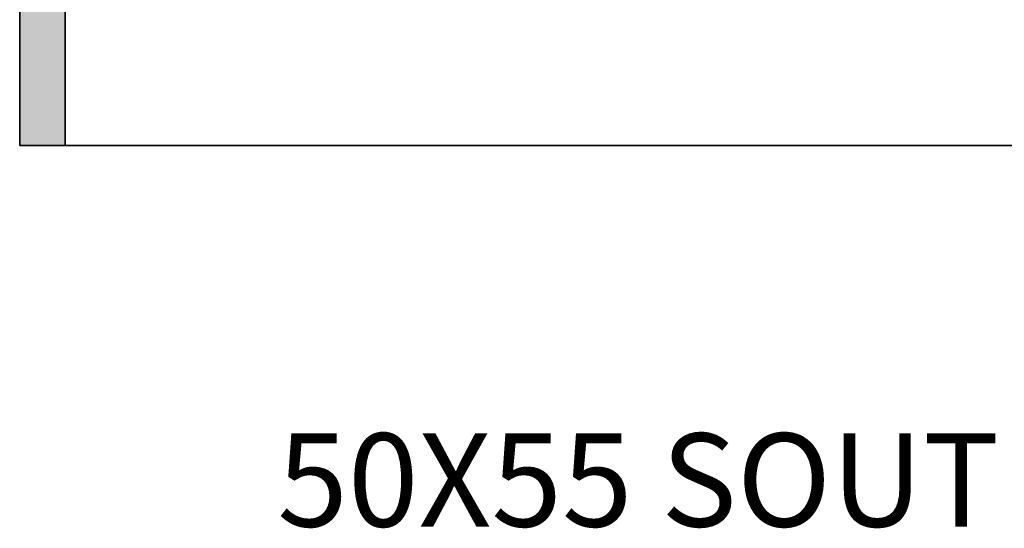
# Model space of a CAD drawing. Units: inches. Extents: x 1319 to 2030, y 219 to 1069.
# Tile 1 of 28: x 1370 to 1565, y 219 to 320. Entities that reach past the tile are written whole.
import ezdxf

# ---------------------------------------------------------------- set-up
doc = ezdxf.new("R2010")
doc.units = ezdxf.units.IN
doc.header["$MEASUREMENT"] = 0
for name, color, linetype, lineweight in [('A-WALL-PATT', 252, 'Continuous', 13), ('C-PROP', 7, 'Continuous', 35), ('text', 7, 'Continuous', 25), ('walls', 250, 'Continuous', 35)]:
    doc.layers.add(name, color=color, linetype=linetype, lineweight=lineweight)
doc.styles.get("Standard").update_dxf_attribs({"font": 'arial.ttf'})

msp = doc.modelspace()

# ---------------------------------------------------------------- hatches: boundary and pattern name
at = {"layer": 'A-WALL-PATT'}
h = msp.add_hatch(color=256, dxfattribs=at)
h.dxf.hatch_style = 1
h.paths.add_polyline_path([(1378.843, 946.227), (1960.843, 946.227), (1960.843, 860.616), (1922.194, 860.616), (1922.194, 851.616), (1960.843, 851.616), (1960.843, 304.227), (1578.343, 304.227), (1578.343, 295.227), (1969.843, 295.227), (1969.843, 955.227), (1369.843, 955.227), (1369.843, 295.227), (1378.843, 295.227)])

# ---------------------------------------------------------------- linework, layer by layer
at = {"layer": 'C-PROP'}
for p, q in [((1369.843, 295.227), (1369.843, 955.227)), ((1969.843, 295.227), (1369.843, 295.227))]:
    msp.add_line(p, q, dxfattribs=at)
at = {"layer": 'walls'}
msp.add_line((1378.843, 295.227), (1378.843, 946.227), dxfattribs=at)

# ---------------------------------------------------------------- texts
at = {"layer": 'text'}
msp.add_text('50X55 SOUTH FACE HOUSE PLAN 3BHK', height=18.48405, dxfattribs=at).set_placement((1420.923, 219.766))

doc.saveas('drawing.dxf')
